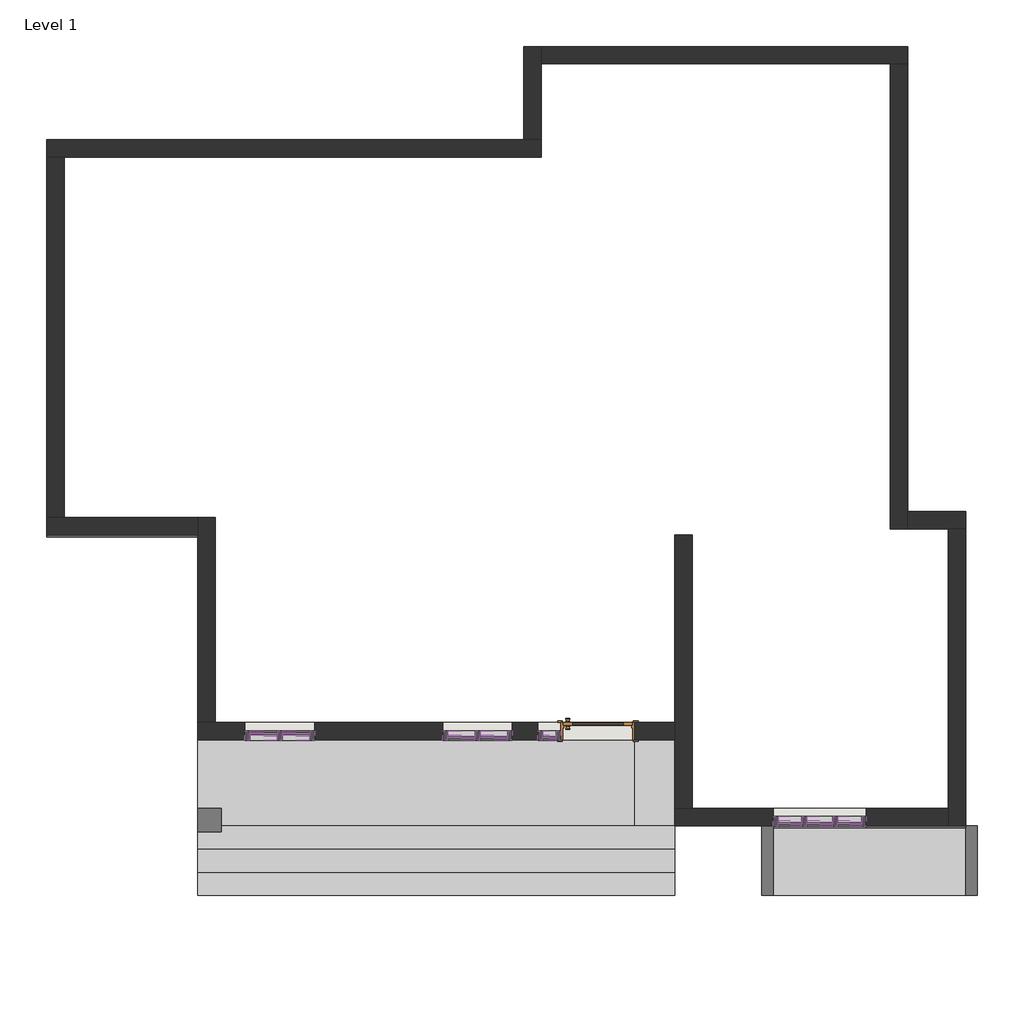
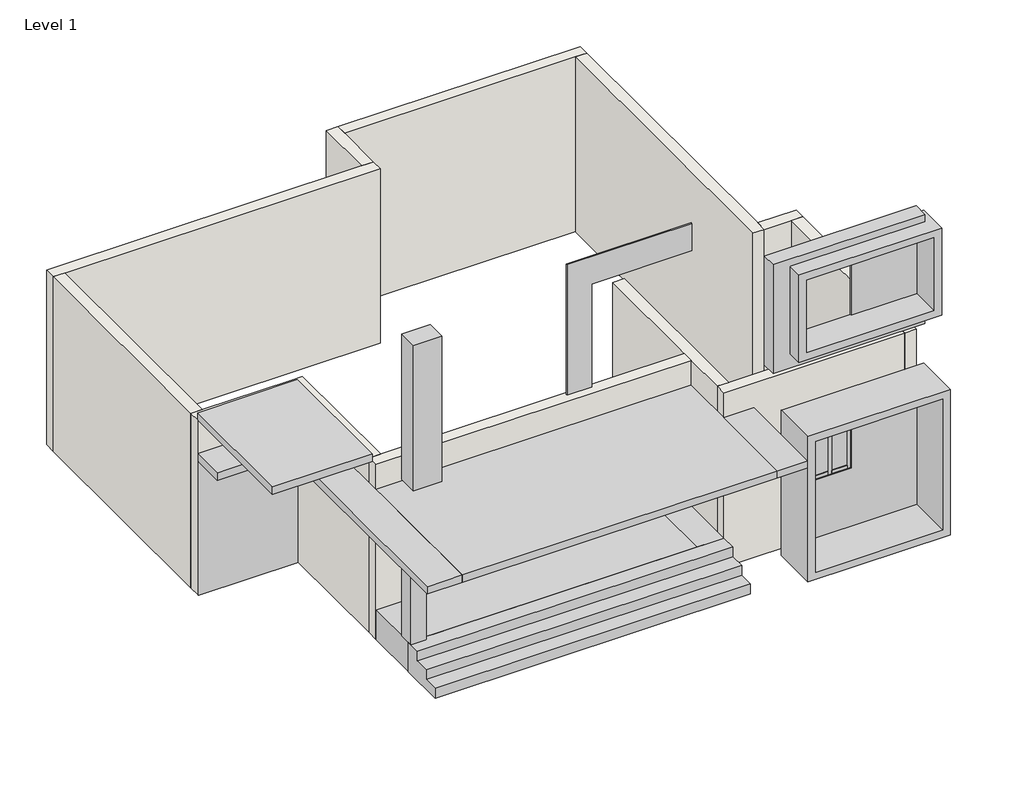
# One storey: 48 members, 16 plates, 12 walls, 1 door, 1 proxy.
"""IFC4 building model written with IfcOpenShell, lengths in millimetres."""

from ifc_helpers import new_model, si_unit, frame, origin, place, context, project, spatial, polyline, outline, extrude, faceted_brep, transform, mapped, element, save
from components import generic_models_1_generic_models_1_206d5355, door_3b97b8e7, member_2344d604, member_a0100b10, member_6c57b699, member_2c71ef08, member_843225dc, member_824a4a8d, member_ffd4c858, member_15823cb3, member_c6627131, member_d92184fb, member_69a911c1, member_f07b7441, member_5ad95953, member_f92b8aa2, member_ff1b7d8f, member_90750a43, member_7fd687a9, member_8e09d03a, system_panel_glazed_8f314941, system_panel_glazed_b220ba01, system_panel_glazed_f8f6f98b, system_panel_glazed_d1623790, system_panel_glazed_0360dae9, system_panel_glazed_809156e5, system_panel_glazed_ff0761ce, system_panel_glazed_bfcc9025

model = new_model("IFC4")

# Units and contexts
model_context = context("Model", 3, world=origin())
ifc_project = project(units=[si_unit("LENGTHUNIT", "METRE", prefix="MILLI")], contexts=[model_context])

# Site, building, storey
site = spatial("IfcSite", under=ifc_project)
building = spatial("IfcBuilding", under=site)
storey = spatial("IfcBuildingStorey", under=building, Name="Level 1", Elevation=0.0)

# Proxy
placement = place(None, origin())
generic_models_1_generic_models_1_shape = generic_models_1_generic_models_1_206d5355(model_context)
element("IfcBuildingElementProxy", 1, Name="Generic Models 1 : Generic Models 1", ObjectType="Generic Models 1 : Generic Models 1", at=placement, inside=storey, context=model_context, shape_type="MappedRepresentation", body=[
    mapped(generic_models_1_generic_models_1_shape, transform((0.0, 0.0, 0.0), x_axis=(1.0, 0.0, 0.0), y_axis=(0.0, 1.0, 0.0), z_axis=(0.0, 0.0, 1.0))),
])

# Door
door_shape = door_3b97b8e7(model_context)
element("IfcDoor", 2, ObjectType="Door-Interior-Single-1_Panel-Wood : 36\" x 84\"", at=placement, inside=storey, context=model_context, shape_type="MappedRepresentation", body=[
    mapped(door_shape, transform((-2625.1415113, 1605.7349631, 0.0), x_axis=(1.0, 0.0, 0.0), y_axis=(0.0, 1.0, 0.0), z_axis=(0.0, 0.0, 1.0))),
])

# Members
member_shape = member_2344d604(model_context)
element("IfcMember", 3, ObjectType="Rectangular Mullion : 1\" Square", at=placement, inside=storey, context=model_context, shape_type="MappedRepresentation", body=[
    mapped(member_shape, transform((-6397.0415113, 1545.4099631, 1676.4), x_axis=(0.0, 0.0, 1.0), y_axis=(0.0, -1.0, 0.0), z_axis=(1.0, 0.0, 0.0))),
])
element("IfcMember", 4, ObjectType="Rectangular Mullion : 1\" Square", at=placement, inside=storey, context=model_context, shape_type="MappedRepresentation", body=[
    mapped(member_shape, transform((-6822.4915113, 1545.4099631, 1676.4), x_axis=(0.0, 0.0, 1.0), y_axis=(0.0, -1.0, 0.0), z_axis=(1.0, 0.0, 0.0))),
])
element("IfcMember", 5, ObjectType="Rectangular Mullion : 1\" Square", at=placement, inside=storey, context=model_context, shape_type="MappedRepresentation", body=[
    mapped(member_shape, transform((-4593.6415113, 1545.4099631, 1676.4), x_axis=(0.0, 0.0, 1.0), y_axis=(0.0, 1.0, 0.0), z_axis=(-1.0, 0.0, 0.0))),
])
element("IfcMember", 6, ObjectType="Rectangular Mullion : 1\" Square", at=placement, inside=storey, context=model_context, shape_type="MappedRepresentation", body=[
    mapped(member_shape, transform((-4168.1915113, 1545.4099631, 1676.4), x_axis=(0.0, 0.0, 1.0), y_axis=(0.0, 1.0, 0.0), z_axis=(-1.0, 0.0, 0.0))),
])
member_2_shape = member_a0100b10(model_context)
element("IfcMember", 7, ObjectType="Rectangular Mullion : 1\" Square", at=placement, inside=storey, context=model_context, shape_type="MappedRepresentation", body=[
    mapped(member_2_shape, transform((-3349.0415113, 1545.4099631, 1701.8), x_axis=(0.0, 0.0, 1.0), y_axis=(0.0, 1.0, 0.0), z_axis=(-1.0, 0.0, 0.0))),
])
member_3_shape = member_6c57b699(model_context)
element("IfcMember", 8, ObjectType="Rectangular Mullion : 1\" Square", at=placement, inside=storey, context=model_context, shape_type="MappedRepresentation", body=[
    mapped(member_3_shape, transform((111.7084887, 421.4599631, 1625.6), x_axis=(0.0, 0.0, 1.0), y_axis=(0.0, 1.0, 0.0), z_axis=(-1.0, 0.0, 0.0))),
])
member_4_shape = member_2c71ef08(model_context)
element("IfcMember", 9, ObjectType="Rectangular Mullion : 1\" Square", at=placement, inside=storey, context=model_context, shape_type="MappedRepresentation", body=[
    mapped(member_4_shape, transform((-262.9415113, 421.4599631, 1625.6), x_axis=(0.0, 0.0, 1.0), y_axis=(0.0, 1.0, 0.0), z_axis=(-1.0, 0.0, 0.0))),
])
element("IfcMember", 10, ObjectType="Rectangular Mullion : 1\" Square", at=placement, inside=storey, context=model_context, shape_type="MappedRepresentation", body=[
    mapped(member_4_shape, transform((518.1084887, 421.4599631, 1625.6), x_axis=(0.0, 0.0, 1.0), y_axis=(0.0, 1.0, 0.0), z_axis=(-1.0, 0.0, 0.0))),
])
member_5_shape = member_843225dc(model_context)
element("IfcMember", 11, ObjectType="Rectangular Mullion : 2.5\" x 5\" rectangular", at=placement, inside=storey, context=model_context, shape_type="MappedRepresentation", body=[
    mapped(member_5_shape, transform((-6397.0415113, 1545.4099631, 2133.6), x_axis=(0.0, 0.0, 1.0), y_axis=(0.0, -1.0, 0.0), z_axis=(1.0, 0.0, 0.0))),
])
element("IfcMember", 12, ObjectType="Rectangular Mullion : 2.5\" x 5\" rectangular", at=placement, inside=storey, context=model_context, shape_type="MappedRepresentation", body=[
    mapped(member_5_shape, transform((-6822.4915113, 1545.4099631, 2133.6), x_axis=(0.0, 0.0, 1.0), y_axis=(0.0, -1.0, 0.0), z_axis=(1.0, 0.0, 0.0))),
])
element("IfcMember", 13, ObjectType="Rectangular Mullion : 2.5\" x 5\" rectangular", at=placement, inside=storey, context=model_context, shape_type="MappedRepresentation", body=[
    mapped(member_5_shape, transform((-4593.6415113, 1545.4099631, 2133.6), x_axis=(0.0, 0.0, 1.0), y_axis=(0.0, 1.0, 0.0), z_axis=(-1.0, 0.0, 0.0))),
])
element("IfcMember", 14, ObjectType="Rectangular Mullion : 2.5\" x 5\" rectangular", at=placement, inside=storey, context=model_context, shape_type="MappedRepresentation", body=[
    mapped(member_5_shape, transform((-4168.1915113, 1545.4099631, 2133.6), x_axis=(0.0, 0.0, 1.0), y_axis=(0.0, 1.0, 0.0), z_axis=(-1.0, 0.0, 0.0))),
])
element("IfcMember", 15, ObjectType="Rectangular Mullion : 2.5\" x 5\" rectangular", at=placement, inside=storey, context=model_context, shape_type="MappedRepresentation", body=[
    mapped(member_5_shape, transform((-7184.4415113, 1545.4099631, 304.8), x_axis=(0.0, 0.0, -1.0), y_axis=(0.0, -1.0, 0.0), z_axis=(-1.0, 0.0, 0.0))),
])
element("IfcMember", 16, ObjectType="Rectangular Mullion : 2.5\" x 5\" rectangular", at=placement, inside=storey, context=model_context, shape_type="MappedRepresentation", body=[
    mapped(member_5_shape, transform((-6758.9915113, 1545.4099631, 304.8), x_axis=(0.0, 0.0, -1.0), y_axis=(0.0, -1.0, 0.0), z_axis=(-1.0, 0.0, 0.0))),
])
element("IfcMember", 17, ObjectType="Rectangular Mullion : 2.5\" x 5\" rectangular", at=placement, inside=storey, context=model_context, shape_type="MappedRepresentation", body=[
    mapped(member_5_shape, transform((-3806.2415113, 1545.4099631, 304.8), x_axis=(0.0, 0.0, -1.0), y_axis=(0.0, 1.0, 0.0), z_axis=(1.0, 0.0, 0.0))),
])
element("IfcMember", 18, ObjectType="Rectangular Mullion : 2.5\" x 5\" rectangular", at=placement, inside=storey, context=model_context, shape_type="MappedRepresentation", body=[
    mapped(member_5_shape, transform((-4231.6915113, 1545.4099631, 304.8), x_axis=(0.0, 0.0, -1.0), y_axis=(0.0, 1.0, 0.0), z_axis=(1.0, 0.0, 0.0))),
])
member_6_shape = member_824a4a8d(model_context)
element("IfcMember", 19, ObjectType="Rectangular Mullion : 2.5\" x 5\" rectangular", at=placement, inside=storey, context=model_context, shape_type="MappedRepresentation", body=[
    mapped(member_6_shape, transform((-6790.7415113, 1545.4099631, 304.8), x_axis=(1.0, 0.0, 0.0), y_axis=(0.0, -1.0, 0.0), z_axis=(0.0, 0.0, -1.0))),
])
element("IfcMember", 20, ObjectType="Rectangular Mullion : 2.5\" x 5\" rectangular", at=placement, inside=storey, context=model_context, shape_type="MappedRepresentation", body=[
    mapped(member_6_shape, transform((-4199.9415113, 1545.4099631, 304.8), x_axis=(-1.0, 0.0, 0.0), y_axis=(0.0, 1.0, 0.0), z_axis=(0.0, 0.0, -1.0))),
])
member_7_shape = member_ffd4c858(model_context)
element("IfcMember", 21, ObjectType="Rectangular Mullion : 2.5\" x 5\" rectangular", at=placement, inside=storey, context=model_context, shape_type="MappedRepresentation", body=[
    mapped(member_7_shape, transform((-6790.7415113, 1545.4099631, 1676.4), x_axis=(1.0, 0.0, 0.0), y_axis=(0.0, -1.0, 0.0), z_axis=(0.0, 0.0, -1.0))),
])
element("IfcMember", 22, ObjectType="Rectangular Mullion : 2.5\" x 5\" rectangular", at=placement, inside=storey, context=model_context, shape_type="MappedRepresentation", body=[
    mapped(member_7_shape, transform((-4199.9415113, 1545.4099631, 1676.4), x_axis=(-1.0, 0.0, 0.0), y_axis=(0.0, 1.0, 0.0), z_axis=(0.0, 0.0, -1.0))),
])
member_8_shape = member_15823cb3(model_context)
element("IfcMember", 23, ObjectType="Rectangular Mullion : 2.5\" x 5\" rectangular", at=placement, inside=storey, context=model_context, shape_type="MappedRepresentation", body=[
    mapped(member_8_shape, transform((-7247.9415113, 1545.4099631, 2133.6), x_axis=(-1.0, 0.0, 0.0), y_axis=(0.0, -1.0, 0.0), z_axis=(0.0, 0.0, 1.0))),
])
element("IfcMember", 24, ObjectType="Rectangular Mullion : 2.5\" x 5\" rectangular", at=placement, inside=storey, context=model_context, shape_type="MappedRepresentation", body=[
    mapped(member_8_shape, transform((-3742.7415113, 1545.4099631, 2133.6), x_axis=(1.0, 0.0, 0.0), y_axis=(0.0, 1.0, 0.0), z_axis=(0.0, 0.0, 1.0))),
])
member_9_shape = member_c6627131(model_context)
element("IfcMember", 25, ObjectType="Rectangular Mullion : 2.5\" x 5\" rectangular", at=placement, inside=storey, context=model_context, shape_type="MappedRepresentation", body=[
    mapped(member_9_shape, transform((-6333.5415113, 1545.4099631, 304.8), x_axis=(1.0, 0.0, 0.0), y_axis=(0.0, -1.0, 0.0), z_axis=(0.0, 0.0, -1.0))),
])
element("IfcMember", 26, ObjectType="Rectangular Mullion : 2.5\" x 5\" rectangular", at=placement, inside=storey, context=model_context, shape_type="MappedRepresentation", body=[
    mapped(member_9_shape, transform((-4657.1415113, 1545.4099631, 304.8), x_axis=(-1.0, 0.0, 0.0), y_axis=(0.0, 1.0, 0.0), z_axis=(0.0, 0.0, -1.0))),
])
element("IfcMember", 27, ObjectType="Rectangular Mullion : 2.5\" x 5\" rectangular", at=placement, inside=storey, context=model_context, shape_type="MappedRepresentation", body=[
    mapped(member_8_shape, transform((-6333.5415113, 1545.4099631, 1676.4), x_axis=(1.0, 0.0, 0.0), y_axis=(0.0, -1.0, 0.0), z_axis=(0.0, 0.0, -1.0))),
])
element("IfcMember", 28, ObjectType="Rectangular Mullion : 2.5\" x 5\" rectangular", at=placement, inside=storey, context=model_context, shape_type="MappedRepresentation", body=[
    mapped(member_8_shape, transform((-4657.1415113, 1545.4099631, 1676.4), x_axis=(-1.0, 0.0, 0.0), y_axis=(0.0, 1.0, 0.0), z_axis=(0.0, 0.0, -1.0))),
])
element("IfcMember", 29, ObjectType="Rectangular Mullion : 2.5\" x 5\" rectangular", at=placement, inside=storey, context=model_context, shape_type="MappedRepresentation", body=[
    mapped(member_9_shape, transform((-7247.9415113, 1545.4099631, 1676.4), x_axis=(-1.0, 0.0, 0.0), y_axis=(0.0, -1.0, 0.0), z_axis=(0.0, 0.0, 1.0))),
])
element("IfcMember", 30, ObjectType="Rectangular Mullion : 2.5\" x 5\" rectangular", at=placement, inside=storey, context=model_context, shape_type="MappedRepresentation", body=[
    mapped(member_9_shape, transform((-3742.7415113, 1545.4099631, 1676.4), x_axis=(1.0, 0.0, 0.0), y_axis=(0.0, 1.0, 0.0), z_axis=(0.0, 0.0, 1.0))),
])
member_10_shape = member_d92184fb(model_context)
element("IfcMember", 31, ObjectType="Rectangular Mullion : 2.5\" x 5\" rectangular", at=placement, inside=storey, context=model_context, shape_type="MappedRepresentation", body=[
    mapped(member_10_shape, transform((-3349.0415113, 1545.4099631, 2133.6), x_axis=(0.0, 0.0, 1.0), y_axis=(0.0, 1.0, 0.0), z_axis=(-1.0, 0.0, 0.0))),
])
element("IfcMember", 32, ObjectType="Rectangular Mullion : 2.5\" x 5\" rectangular", at=placement, inside=storey, context=model_context, shape_type="MappedRepresentation", body=[
    mapped(member_10_shape, transform((-3171.2415113, 1545.4099631, 304.8), x_axis=(0.0, 0.0, -1.0), y_axis=(0.0, 1.0, 0.0), z_axis=(1.0, 0.0, 0.0))),
])
member_11_shape = member_69a911c1(model_context)
element("IfcMember", 33, ObjectType="Rectangular Mullion : 2.5\" x 5\" rectangular", at=placement, inside=storey, context=model_context, shape_type="MappedRepresentation", body=[
    mapped(member_11_shape, transform((-3107.7415113, 1545.4099631, 2133.6), x_axis=(1.0, 0.0, 0.0), y_axis=(0.0, 1.0, 0.0), z_axis=(0.0, 0.0, 1.0))),
])
member_12_shape = member_f07b7441(model_context)
element("IfcMember", 34, ObjectType="Rectangular Mullion : 2.5\" x 5\" rectangular", at=placement, inside=storey, context=model_context, shape_type="MappedRepresentation", body=[
    mapped(member_12_shape, transform((-3412.5415113, 1545.4099631, 304.8), x_axis=(-1.0, 0.0, 0.0), y_axis=(0.0, 1.0, 0.0), z_axis=(0.0, 0.0, -1.0))),
])
element("IfcMember", 35, ObjectType="Rectangular Mullion : 2.5\" x 5\" rectangular", at=placement, inside=storey, context=model_context, shape_type="MappedRepresentation", body=[
    mapped(member_11_shape, transform((-3412.5415113, 1545.4099631, 1701.8), x_axis=(-1.0, 0.0, 0.0), y_axis=(0.0, 1.0, 0.0), z_axis=(0.0, 0.0, -1.0))),
])
element("IfcMember", 36, ObjectType="Rectangular Mullion : 2.5\" x 5\" rectangular", at=placement, inside=storey, context=model_context, shape_type="MappedRepresentation", body=[
    mapped(member_12_shape, transform((-3107.7415113, 1545.4099631, 1701.8), x_axis=(1.0, 0.0, 0.0), y_axis=(0.0, 1.0, 0.0), z_axis=(0.0, 0.0, 1.0))),
])
member_13_shape = member_5ad95953(model_context)
element("IfcMember", 37, ObjectType="Rectangular Mullion : 2.5\" x 5\" rectangular", at=placement, inside=storey, context=model_context, shape_type="MappedRepresentation", body=[
    mapped(member_13_shape, transform((-262.9415113, 421.4599631, 2133.6), x_axis=(0.0, 0.0, 1.0), y_axis=(0.0, 1.0, 0.0), z_axis=(-1.0, 0.0, 0.0))),
])
element("IfcMember", 38, ObjectType="Rectangular Mullion : 2.5\" x 5\" rectangular", at=placement, inside=storey, context=model_context, shape_type="MappedRepresentation", body=[
    mapped(member_13_shape, transform((518.1084887, 421.4599631, 2133.6), x_axis=(0.0, 0.0, 1.0), y_axis=(0.0, 1.0, 0.0), z_axis=(-1.0, 0.0, 0.0))),
])
element("IfcMember", 39, ObjectType="Rectangular Mullion : 2.5\" x 5\" rectangular", at=placement, inside=storey, context=model_context, shape_type="MappedRepresentation", body=[
    mapped(member_13_shape, transform((829.2584887, 421.4599631, 609.6), x_axis=(0.0, 0.0, -1.0), y_axis=(0.0, 1.0, 0.0), z_axis=(1.0, 0.0, 0.0))),
])
element("IfcMember", 40, ObjectType="Rectangular Mullion : 2.5\" x 5\" rectangular", at=placement, inside=storey, context=model_context, shape_type="MappedRepresentation", body=[
    mapped(member_13_shape, transform((48.2084887, 421.4599631, 609.6), x_axis=(0.0, 0.0, -1.0), y_axis=(0.0, 1.0, 0.0), z_axis=(1.0, 0.0, 0.0))),
])
member_14_shape = member_f92b8aa2(model_context)
element("IfcMember", 41, ObjectType="Rectangular Mullion : 2.5\" x 5\" rectangular", at=placement, inside=storey, context=model_context, shape_type="MappedRepresentation", body=[
    mapped(member_14_shape, transform((79.9584887, 421.4599631, 609.6), x_axis=(-1.0, 0.0, 0.0), y_axis=(0.0, 1.0, 0.0), z_axis=(0.0, 0.0, -1.0))),
])
element("IfcMember", 42, ObjectType="Rectangular Mullion : 2.5\" x 5\" rectangular", at=placement, inside=storey, context=model_context, shape_type="MappedRepresentation", body=[
    mapped(member_14_shape, transform((486.3584887, 421.4599631, 609.6), x_axis=(-1.0, 0.0, 0.0), y_axis=(0.0, 1.0, 0.0), z_axis=(0.0, 0.0, -1.0))),
])
member_15_shape = member_ff1b7d8f(model_context)
element("IfcMember", 43, ObjectType="Rectangular Mullion : 2.5\" x 5\" rectangular", at=placement, inside=storey, context=model_context, shape_type="MappedRepresentation", body=[
    mapped(member_15_shape, transform((454.6084887, 421.4599631, 609.6), x_axis=(0.0, 0.0, -1.0), y_axis=(0.0, 1.0, 0.0), z_axis=(1.0, 0.0, 0.0))),
])
element("IfcMember", 44, ObjectType="Rectangular Mullion : 2.5\" x 5\" rectangular", at=placement, inside=storey, context=model_context, shape_type="MappedRepresentation", body=[
    mapped(member_15_shape, transform((111.7084887, 421.4599631, 2133.6), x_axis=(0.0, 0.0, 1.0), y_axis=(0.0, 1.0, 0.0), z_axis=(-1.0, 0.0, 0.0))),
])
member_16_shape = member_90750a43(model_context)
element("IfcMember", 45, ObjectType="Rectangular Mullion : 2.5\" x 5\" rectangular", at=placement, inside=storey, context=model_context, shape_type="MappedRepresentation", body=[
    mapped(member_16_shape, transform((79.9584887, 421.4599631, 1625.6), x_axis=(-1.0, 0.0, 0.0), y_axis=(0.0, 1.0, 0.0), z_axis=(0.0, 0.0, -1.0))),
])
element("IfcMember", 46, ObjectType="Rectangular Mullion : 2.5\" x 5\" rectangular", at=placement, inside=storey, context=model_context, shape_type="MappedRepresentation", body=[
    mapped(member_16_shape, transform((486.3584887, 421.4599631, 1625.6), x_axis=(-1.0, 0.0, 0.0), y_axis=(0.0, 1.0, 0.0), z_axis=(0.0, 0.0, -1.0))),
])
member_17_shape = member_7fd687a9(model_context)
element("IfcMember", 47, ObjectType="Rectangular Mullion : 2.5\" x 5\" rectangular", at=placement, inside=storey, context=model_context, shape_type="MappedRepresentation", body=[
    mapped(member_17_shape, transform((892.7584887, 421.4599631, 2133.6), x_axis=(1.0, 0.0, 0.0), y_axis=(0.0, 1.0, 0.0), z_axis=(0.0, 0.0, 1.0))),
])
member_18_shape = member_8e09d03a(model_context)
element("IfcMember", 48, ObjectType="Rectangular Mullion : 2.5\" x 5\" rectangular", at=placement, inside=storey, context=model_context, shape_type="MappedRepresentation", body=[
    mapped(member_18_shape, transform((-326.4415113, 421.4599631, 609.6), x_axis=(-1.0, 0.0, 0.0), y_axis=(0.0, 1.0, 0.0), z_axis=(0.0, 0.0, -1.0))),
])
element("IfcMember", 49, ObjectType="Rectangular Mullion : 2.5\" x 5\" rectangular", at=placement, inside=storey, context=model_context, shape_type="MappedRepresentation", body=[
    mapped(member_17_shape, transform((-326.4415113, 421.4599631, 1625.6), x_axis=(-1.0, 0.0, 0.0), y_axis=(0.0, 1.0, 0.0), z_axis=(0.0, 0.0, -1.0))),
])
element("IfcMember", 50, ObjectType="Rectangular Mullion : 2.5\" x 5\" rectangular", at=placement, inside=storey, context=model_context, shape_type="MappedRepresentation", body=[
    mapped(member_18_shape, transform((892.7584887, 421.4599631, 1625.6), x_axis=(1.0, 0.0, 0.0), y_axis=(0.0, 1.0, 0.0), z_axis=(0.0, 0.0, 1.0))),
])

# Plates
system_panel_glazed_shape = system_panel_glazed_8f314941(model_context)
element("IfcPlate", 51, ObjectType="System Panel : Glazed", at=placement, inside=storey, context=model_context, shape_type="MappedRepresentation", body=[
    mapped(system_panel_glazed_shape, transform((-3987.2165113, 1545.4099631, 368.3), x_axis=(-1.0, 0.0, 0.0), y_axis=(0.0, -1.0, 0.0), z_axis=(0.0, 0.0, 1.0))),
])
element("IfcPlate", 52, ObjectType="System Panel : Glazed", at=placement, inside=storey, context=model_context, shape_type="MappedRepresentation", body=[
    mapped(system_panel_glazed_shape, transform((-7003.4665113, 1545.4099631, 368.3), x_axis=(1.0, 0.0, 0.0), y_axis=(0.0, 1.0, 0.0), z_axis=(0.0, 0.0, 1.0))),
])
element("IfcPlate", 53, ObjectType="System Panel : Glazed", at=placement, inside=storey, context=model_context, shape_type="MappedRepresentation", body=[
    mapped(system_panel_glazed_shape, transform((-6578.0165113, 1545.4099631, 368.3), x_axis=(1.0, 0.0, 0.0), y_axis=(0.0, 1.0, 0.0), z_axis=(0.0, 0.0, 1.0))),
])
element("IfcPlate", 54, ObjectType="System Panel : Glazed", at=placement, inside=storey, context=model_context, shape_type="MappedRepresentation", body=[
    mapped(system_panel_glazed_shape, transform((-4412.6665113, 1545.4099631, 368.3), x_axis=(-1.0, 0.0, 0.0), y_axis=(0.0, -1.0, 0.0), z_axis=(0.0, 0.0, 1.0))),
])
system_panel_glazed_2_shape = system_panel_glazed_b220ba01(model_context)
element("IfcPlate", 55, ObjectType="System Panel : Glazed", at=placement, inside=storey, context=model_context, shape_type="MappedRepresentation", body=[
    mapped(system_panel_glazed_2_shape, transform((-7003.4665113, 1545.4099631, 1676.4), x_axis=(1.0, 0.0, 0.0), y_axis=(0.0, 1.0, 0.0), z_axis=(0.0, 0.0, 1.0))),
])
element("IfcPlate", 56, ObjectType="System Panel : Glazed", at=placement, inside=storey, context=model_context, shape_type="MappedRepresentation", body=[
    mapped(system_panel_glazed_2_shape, transform((-6578.0165113, 1545.4099631, 1676.4), x_axis=(1.0, 0.0, 0.0), y_axis=(0.0, 1.0, 0.0), z_axis=(0.0, 0.0, 1.0))),
])
element("IfcPlate", 57, ObjectType="System Panel : Glazed", at=placement, inside=storey, context=model_context, shape_type="MappedRepresentation", body=[
    mapped(system_panel_glazed_2_shape, transform((-3987.2165113, 1545.4099631, 1676.4), x_axis=(-1.0, 0.0, 0.0), y_axis=(0.0, -1.0, 0.0), z_axis=(0.0, 0.0, 1.0))),
])
element("IfcPlate", 58, ObjectType="System Panel : Glazed", at=placement, inside=storey, context=model_context, shape_type="MappedRepresentation", body=[
    mapped(system_panel_glazed_2_shape, transform((-4412.6665113, 1545.4099631, 1676.4), x_axis=(-1.0, 0.0, 0.0), y_axis=(0.0, -1.0, 0.0), z_axis=(0.0, 0.0, 1.0))),
])
system_panel_glazed_3_shape = system_panel_glazed_f8f6f98b(model_context)
element("IfcPlate", 59, ObjectType="System Panel : Glazed", at=placement, inside=storey, context=model_context, shape_type="MappedRepresentation", body=[
    mapped(system_panel_glazed_3_shape, transform((-3260.1415113, 1545.4099631, 368.3), x_axis=(-1.0, 0.0, 0.0), y_axis=(0.0, -1.0, 0.0), z_axis=(0.0, 0.0, 1.0))),
])
system_panel_glazed_4_shape = system_panel_glazed_d1623790(model_context)
element("IfcPlate", 60, ObjectType="System Panel : Glazed", at=placement, inside=storey, context=model_context, shape_type="MappedRepresentation", body=[
    mapped(system_panel_glazed_4_shape, transform((-3260.1415113, 1545.4099631, 1701.8), x_axis=(-1.0, 0.0, 0.0), y_axis=(0.0, -1.0, 0.0), z_axis=(0.0, 0.0, 1.0))),
])
system_panel_glazed_5_shape = system_panel_glazed_0360dae9(model_context)
element("IfcPlate", 61, ObjectType="System Panel : Glazed", at=placement, inside=storey, context=model_context, shape_type="MappedRepresentation", body=[
    mapped(system_panel_glazed_5_shape, transform((673.6834887, 421.4599631, 673.1), x_axis=(-1.0, 0.0, 0.0), y_axis=(0.0, -1.0, 0.0), z_axis=(0.0, 0.0, 1.0))),
])
element("IfcPlate", 62, ObjectType="System Panel : Glazed", at=placement, inside=storey, context=model_context, shape_type="MappedRepresentation", body=[
    mapped(system_panel_glazed_5_shape, transform((-107.3665113, 421.4599631, 673.1), x_axis=(-1.0, 0.0, 0.0), y_axis=(0.0, -1.0, 0.0), z_axis=(0.0, 0.0, 1.0))),
])
system_panel_glazed_6_shape = system_panel_glazed_809156e5(model_context)
element("IfcPlate", 63, ObjectType="System Panel : Glazed", at=placement, inside=storey, context=model_context, shape_type="MappedRepresentation", body=[
    mapped(system_panel_glazed_6_shape, transform((283.1584887, 421.4599631, 673.1), x_axis=(-1.0, 0.0, 0.0), y_axis=(0.0, -1.0, 0.0), z_axis=(0.0, 0.0, 1.0))),
])
system_panel_glazed_7_shape = system_panel_glazed_ff0761ce(model_context)
element("IfcPlate", 64, ObjectType="System Panel : Glazed", at=placement, inside=storey, context=model_context, shape_type="MappedRepresentation", body=[
    mapped(system_panel_glazed_7_shape, transform((673.6834887, 421.4599631, 1625.6), x_axis=(-1.0, 0.0, 0.0), y_axis=(0.0, -1.0, 0.0), z_axis=(0.0, 0.0, 1.0))),
])
element("IfcPlate", 65, ObjectType="System Panel : Glazed", at=placement, inside=storey, context=model_context, shape_type="MappedRepresentation", body=[
    mapped(system_panel_glazed_7_shape, transform((-107.3665113, 421.4599631, 1625.6), x_axis=(-1.0, 0.0, 0.0), y_axis=(0.0, -1.0, 0.0), z_axis=(0.0, 0.0, 1.0))),
])
system_panel_glazed_8_shape = system_panel_glazed_bfcc9025(model_context)
element("IfcPlate", 66, ObjectType="System Panel : Glazed", at=placement, inside=storey, context=model_context, shape_type="MappedRepresentation", body=[
    mapped(system_panel_glazed_8_shape, transform((283.1584887, 421.4599631, 1625.6), x_axis=(-1.0, 0.0, 0.0), y_axis=(0.0, -1.0, 0.0), z_axis=(0.0, 0.0, 1.0))),
])

# Walls
element("IfcWall", 67, ObjectType="9\" wall", at=placement, inside=storey, context=model_context, shape_type="Brep", body=[
    faceted_brep([(-9845.0915113, 9127.3099631, -609.6), (-9616.4915113, 9127.3099631, -609.6), (-3368.0915113, 9127.3099631, -609.6), (-3368.0915113, 9127.3099631, 3048.0), (-9616.4915113, 9127.3099631, 3048.0), (-9845.0915113, 9127.3099631, 3048.0), (-9845.0915113, 9355.9099631, -609.6), (-9845.0915113, 9355.9099631, 3048.0), (-3596.6915113, 9355.9099631, 3048.0), (-3368.0915113, 9355.9099631, 3048.0), (-3368.0915113, 9355.9099631, -609.6), (-3596.6915113, 9355.9099631, -609.6)], [[[0, 1, 2, 3, 4, 5]], [[6, 7, 8, 9, 10, 11]], [[2, 1, 0, 6, 11, 10]], [[5, 4, 3, 9, 8, 7]], [[3, 2, 10, 9]], [[0, 5, 7, 6]]]),
])
element("IfcWall", 68, ObjectType="9\" wall", at=placement, inside=storey, context=model_context, shape_type="Brep", body=[
    faceted_brep([(-3368.0915113, 9355.9099631, -609.6), (-3368.0915113, 10346.5099631, -609.6), (-3368.0915113, 10575.1099631, -609.6), (-3368.0915113, 10575.1099631, 3048.0), (-3368.0915113, 10346.5099631, 3048.0), (-3368.0915113, 9355.9099631, 3048.0), (-3596.6915113, 9355.9099631, -609.6), (-3596.6915113, 9355.9099631, 3048.0), (-3596.6915113, 10575.1099631, 3048.0), (-3596.6915113, 10575.1099631, -609.6)], [[[0, 1, 2, 3, 4, 5]], [[6, 7, 8, 9]], [[2, 1, 0, 6, 9]], [[5, 4, 3, 8, 7]], [[0, 5, 7, 6]], [[3, 2, 9, 8]]]),
])
element("IfcWall", 69, ObjectType="9\" wall", at=placement, inside=storey, context=model_context, shape_type="Brep", body=[
    faceted_brep([(-3368.0915113, 10346.5099631, -609.6), (1203.9084887, 10346.5099631, -609.6), (1432.5084887, 10346.5099631, -609.6), (1432.5084887, 10346.5099631, 3048.0), (1203.9084887, 10346.5099631, 3048.0), (-3368.0915113, 10346.5099631, 3048.0), (-3368.0915113, 10575.1099631, -609.6), (-3368.0915113, 10575.1099631, 3048.0), (1432.5084887, 10575.1099631, 3048.0), (1432.5084887, 10575.1099631, -609.6)], [[[0, 1, 2, 3, 4, 5]], [[6, 7, 8, 9]], [[2, 1, 0, 6, 9]], [[5, 4, 3, 8, 7]], [[0, 5, 7, 6]], [[3, 2, 9, 8]]]),
])
element("IfcWall", 70, ObjectType="9\" wall", at=placement, inside=storey, context=model_context, shape_type="Brep", body=[
    faceted_brep([(1203.9084887, 10346.5099631, -609.6), (1203.9084887, 4250.5099631, -609.6), (1203.9084887, 4250.5099631, 3048.0), (1203.9084887, 10346.5099631, 3048.0), (1432.5084887, 10346.5099631, -609.6), (1432.5084887, 10346.5099631, 3048.0), (1432.5084887, 4479.1099631, 3048.0), (1432.5084887, 4250.5099631, 3048.0), (1432.5084887, 4250.5099631, -609.6), (1432.5084887, 4479.1099631, -609.6)], [[[0, 1, 2, 3]], [[4, 5, 6, 7, 8, 9]], [[1, 0, 4, 9, 8]], [[3, 2, 7, 6, 5]], [[0, 3, 5, 4]], [[2, 1, 8, 7]]]),
])
element("IfcWall", 71, ObjectType="9\" wall", at=placement, inside=storey, context=model_context, shape_type="Brep", body=[
    faceted_brep([(1432.5084887, 4250.5099631, -609.6), (1965.9084887, 4250.5099631, -609.6), (2194.5084887, 4250.5099631, -609.6), (2194.5084887, 4250.5099631, 3048.0), (1965.9084887, 4250.5099631, 3048.0), (1432.5084887, 4250.5099631, 3048.0), (1432.5084887, 4479.1099631, -609.6), (1432.5084887, 4479.1099631, 3048.0), (2194.5084887, 4479.1099631, 3048.0), (2194.5084887, 4479.1099631, -609.6)], [[[0, 1, 2, 3, 4, 5]], [[6, 7, 8, 9]], [[2, 1, 0, 6, 9]], [[5, 4, 3, 8, 7]], [[0, 5, 7, 6]], [[3, 2, 9, 8]]]),
])
element("IfcWall", 72, ObjectType="9\" wall", at=placement, inside=storey, context=model_context, shape_type="Brep", body=[
    faceted_brep([(1965.9084887, 4250.5099631, -609.6), (1965.9084887, 592.9099631, -609.6), (1965.9084887, 364.3099631, -609.6), (1965.9084887, 364.3099631, 3048.0), (1965.9084887, 592.9099631, 3048.0), (1965.9084887, 4250.5099631, 3048.0), (2194.5084887, 4250.5099631, -609.6), (2194.5084887, 4250.5099631, 3048.0), (2194.5084887, 364.3099631, 3048.0), (2194.5084887, 364.3099631, -609.6)], [[[0, 1, 2, 3, 4, 5]], [[6, 7, 8, 9]], [[2, 1, 0, 6, 9]], [[5, 4, 3, 8, 7]], [[0, 5, 7, 6]], [[3, 2, 9, 8]]]),
])
element("IfcWall", 73, ObjectType="9\" wall", at=placement, inside=storey, context=model_context, shape_type="Brep", body=[
    faceted_brep([(1965.9084887, 592.9099631, -609.6), (-1386.8915113, 592.9099631, -609.6), (-1615.4915113, 592.9099631, -609.6), (-1615.4915113, 592.9099631, 3048.0), (-1386.8915113, 592.9099631, 3048.0), (1965.9084887, 592.9099631, 3048.0), (892.7584887, 592.9099631, 609.6), (892.7584887, 592.9099631, 2133.6), (-326.4415113, 592.9099631, 2133.6), (-326.4415113, 592.9099631, 609.6), (-1615.4915113, 364.3099631, -609.6), (1965.9084887, 364.3099631, -609.6), (1965.9084887, 364.3099631, 3048.0), (-1615.4915113, 364.3099631, 3048.0), (-1615.4915113, 364.3099631, 2530.5713747), (892.7584887, 364.3099631, 2133.6), (892.7584887, 364.3099631, 609.6), (-326.4415113, 364.3099631, 609.6), (-326.4415113, 364.3099631, 2133.6)], [[[0, 1, 2, 3, 4, 5], [6, 7, 8, 9]], [[10, 11, 12, 13, 14], [15, 16, 17, 18]], [[2, 1, 0, 11, 10]], [[5, 4, 3, 13, 12]], [[0, 5, 12, 11]], [[6, 16, 15, 7]], [[7, 15, 18, 8]], [[8, 18, 17, 9]], [[16, 6, 9, 17]], [[2, 10, 14, 13, 3]]]),
])
element("IfcWall", 74, ObjectType="9\" wall", at=placement, inside=storey, context=model_context, shape_type="Brep", body=[
    faceted_brep([(-1386.8915113, 592.9099631, 3048.0), (-1386.8915113, 592.9099631, -609.6), (-1386.8915113, 4174.3099631, -609.6), (-1386.8915113, 4174.3099631, 3048.0), (-1615.4915113, 592.9099631, -609.6), (-1615.4915113, 592.9099631, 3048.0), (-1615.4915113, 1488.2599631, 3048.0), (-1615.4915113, 1716.8599631, 3048.0), (-1615.4915113, 4174.3099631, 3048.0), (-1615.4915113, 4174.3099631, -609.6), (-1615.4915113, 1716.8599631, -609.6), (-1615.4915113, 1488.2599631, -609.6)], [[[0, 1, 2, 3]], [[4, 5, 6, 7, 8, 9, 10, 11]], [[2, 1, 4, 11, 10, 9]], [[3, 2, 9, 8]], [[0, 3, 8, 7, 6, 5]], [[0, 5, 4, 1]]]),
])
element("IfcWall", 75, ObjectType="9\" wall", at=placement, inside=storey, context=model_context, shape_type="Brep", body=[
    faceted_brep([(-1615.4915113, 1716.8599631, -609.6), (-7635.2915113, 1716.8599631, -609.6), (-7863.8915113, 1716.8599631, -609.6), (-7863.8915113, 1716.8599631, 3048.0), (-7635.2915113, 1716.8599631, 3048.0), (-1615.4915113, 1716.8599631, 3048.0), (-2142.5415113, 1716.8599631, 0.0), (-2142.5415113, 1716.8599631, 2159.0), (-3107.7415113, 1716.8599631, 2159.0), (-3107.7415113, 1716.8599631, 2133.6), (-3412.5415113, 1716.8599631, 2133.6), (-3412.5415113, 1716.8599631, 304.8), (-3107.7415113, 1716.8599631, 304.8), (-3107.7415113, 1716.8599631, 0.0), (-7247.9415113, 1716.8599631, 2133.6), (-7247.9415113, 1716.8599631, 304.8), (-6333.5415113, 1716.8599631, 304.8), (-6333.5415113, 1716.8599631, 2133.6), (-3742.7415113, 1716.8599631, 304.8), (-3742.7415113, 1716.8599631, 2133.6), (-4657.1415113, 1716.8599631, 2133.6), (-4657.1415113, 1716.8599631, 304.8), (-7863.8915113, 1488.2599631, -609.6), (-1615.4915113, 1488.2599631, -609.6), (-1615.4915113, 1488.2599631, 3048.0), (-7863.8915113, 1488.2599631, 3048.0), (-7863.8915113, 1488.2599631, 2530.5713747), (-2142.5415113, 1488.2599631, 2159.0), (-2142.5415113, 1488.2599631, 0.0), (-3107.7415113, 1488.2599631, 0.0), (-3107.7415113, 1488.2599631, 304.8), (-3412.5415113, 1488.2599631, 304.8), (-3412.5415113, 1488.2599631, 2133.6), (-3107.7415113, 1488.2599631, 2133.6), (-3107.7415113, 1488.2599631, 2159.0), (-7247.9415113, 1488.2599631, 304.8), (-7247.9415113, 1488.2599631, 2133.6), (-6333.5415113, 1488.2599631, 2133.6), (-6333.5415113, 1488.2599631, 304.8), (-3742.7415113, 1488.2599631, 2133.6), (-3742.7415113, 1488.2599631, 304.8), (-4657.1415113, 1488.2599631, 304.8), (-4657.1415113, 1488.2599631, 2133.6)], [[[0, 1, 2, 3, 4, 5], [6, 7, 8, 9, 10, 11, 12, 13], [14, 15, 16, 17], [18, 19, 20, 21]], [[22, 23, 24, 25, 26], [27, 28, 29, 30, 31, 32, 33, 34], [35, 36, 37, 38], [39, 40, 41, 42]], [[2, 1, 0, 23, 22]], [[5, 4, 3, 25, 24]], [[0, 5, 24, 23]], [[6, 28, 27, 7]], [[7, 27, 34, 8]], [[29, 13, 12, 30]], [[8, 34, 33, 9]], [[28, 6, 13, 29]], [[35, 15, 14, 36]], [[36, 14, 17, 37]], [[37, 17, 16, 38]], [[15, 35, 38, 16]], [[39, 19, 18, 40]], [[19, 39, 42, 20]], [[20, 42, 41, 21]], [[40, 18, 21, 41]], [[32, 10, 9, 33]], [[10, 32, 31, 11]], [[11, 31, 30, 12]], [[2, 22, 26, 25, 3]]]),
])
element("IfcWall", 76, ObjectType="9\" wall", at=placement, inside=storey, context=model_context, shape_type="Brep", body=[
    faceted_brep([(-7635.2915113, 1716.8599631, 3048.0), (-7635.2915113, 1716.8599631, -609.6), (-7635.2915113, 4402.9099631, -609.6), (-7635.2915113, 4402.9099631, 3048.0), (-7863.8915113, 1716.8599631, -609.6), (-7863.8915113, 1716.8599631, 3048.0), (-7863.8915113, 4174.3099631, 3048.0), (-7863.8915113, 4402.9099631, 3048.0), (-7863.8915113, 4402.9099631, -609.6), (-7863.8915113, 4174.3099631, -609.6)], [[[0, 1, 2, 3]], [[4, 5, 6, 7, 8, 9]], [[2, 1, 4, 9, 8]], [[0, 3, 7, 6, 5]], [[3, 2, 8, 7]], [[0, 5, 4, 1]]]),
])
element("IfcWall", 77, ObjectType="9\" wall", at=placement, inside=storey, context=model_context, shape_type="Brep", body=[
    faceted_brep([(-7863.8915113, 4402.9099631, -609.6), (-9616.4915113, 4402.9099631, -609.6), (-9845.0915113, 4402.9099631, -609.6), (-9845.0915113, 4402.9099631, 3048.0), (-9616.4915113, 4402.9099631, 3048.0), (-7863.8915113, 4402.9099631, 3048.0), (-7863.8915113, 4174.3099631, -609.6), (-7863.8915113, 4174.3099631, 3048.0), (-9845.0915113, 4174.3099631, 3048.0), (-9845.0915113, 4174.3099631, -609.6)], [[[0, 1, 2, 3, 4, 5]], [[6, 7, 8, 9]], [[2, 1, 0, 6, 9]], [[5, 4, 3, 8, 7]], [[0, 5, 7, 6]], [[3, 2, 9, 8]]]),
])
element("IfcWall", 78, ObjectType="9\" wall", at=placement, inside=storey, context=model_context, shape_type="SweptSolid", body=[
    extrude(outline(polyline([(-9616.4915113, 9127.3099631), (-9616.4915113, 4402.9099631), (-9845.0915113, 4402.9099631), (-9845.0915113, 9127.3099631), (-9616.4915113, 9127.3099631)])), frame((0.0, 0.0, -609.6), z_axis=(0.0, 0.0, 1.0), x_axis=(1.0, 0.0, 0.0)), (0.0, 0.0, 1.0), 3657.6),
])

save(model, "model.ifc")

# Revit data of these elements
# Type "Door-Interior-Single-1_Panel-Wood : 36\" x 84\""
#   Type Mark = "8"
#   Assembly Code = "C1020300"
#   Analytic Construction = "Wooden"
#   Top Rail = 0' - 4 11/16"
#   Thickness = 0' - 1 3/8"
#   Thermal Resistance (R) = 2.5876 (h·ft²·°F)/BTU
#   Swing Angle [instance default] = 90.00°
#   Stiles = 0' - 4 3/4"
#   Rough Width = 3' - 2"
#   Rough Height = 7' - 1"
#   Height = 7' - 0"
#   Width = 3' - 0"
#   Heat Transfer Coefficient (U) = 0.3865 BTU/(h·ft²·°F)
#   Bottom Rail = 0' - 9 1/8"
#   Trim Material = Cherry
#   Panel Material = Cherry
#   Frame Material = Cherry
#   Door Handle Material = Aluminum
#   Visual Light Transmittance = 0
#   Solar Heat Gain Coefficient = 0
#   Wall Closure = (empty or 0)
#   Function = (empty or 0)
# Type "Rectangular Mullion : 1\" Square"
#   built-in parameter 1007304 = 0.0833333 (stored number, unit not read)
#   built-in parameter 1007301 = 0.0416667 (stored number, unit not read)
#   built-in parameter 1007300 = 0.0416667 (stored number, unit not read)
# Type "Rectangular Mullion : 2.5\" x 5\" rectangular"
#   built-in parameter 1007304 = 0.416667 (stored number, unit not read)
#   built-in parameter 1007301 = 0.104167 (stored number, unit not read)
#   built-in parameter 1007300 = 0.104167 (stored number, unit not read)
# Type "System Panel : Glazed"
#   Construction Type Id = "GSP4R"
#   Analytic Construction = "1/8 in Pilkington single glazing"
#   Visual Light Transmittance = 0.9
#   Solar Heat Gain Coefficient = 0.86
#   Heat Transfer Coefficient (U) = 1.18115 BTU/(h·ft²·°F)
#   Define Thermal Properties by = 1
# Type "9\" wall"
#   Assembly Code = "B2010"
#   Layers, outside or top first: 0' - 9" "Laminate, Ivory, Matte" (function 1)
# Element 1 (IfcBuildingElementProxy, "Generic Models 1 : Generic Models 1")
#   Phase Created = New Construction
#   Materials on its faces: "Laminate, Ivory, Matte", "Wood Planks"
# Element 2 (IfcDoor, "Door-Interior-Single-1_Panel-Wood : 36\" x 84\"")
#   Swing Angle = 90.00°
#   Phase Created = New Construction
#   Materials on its faces: "Cherry", "Aluminum"
# Elements 3, 4, 5, 6, 7, 8, 9, 10 (IfcMember, "Rectangular Mullion : 1\" Square")
#   Phase Created = New Construction
# Elements 11, 12, 13, 14, 15, 16, 17, 18, 19, 20, 21, 22, 23, 24, 25, 26, 27, 28, 29, 30, 31, 32, 33, 34, 35, 36, 37, 38, 39, 40, 41, 42, 43, 44, 45, 46, 47, 48, 49, 50 (IfcMember, "Rectangular Mullion : 2.5\" x 5\" rectangular")
#   Phase Created = New Construction
# Elements 51, 52, 53, 54, 55, 56, 57, 58, 59, 60, 61, 62, 63, 64, 65, 66 (IfcPlate, "System Panel : Glazed")
#   Phase Created = New Construction
#   Materials on its faces: "Glass"
# Elements 67, 68, 69, 70, 71, 72, 73, 74, 75, 76, 77, 78 (IfcWall, "9\" wall")
#   built-in parameter 1001111 = -2' - 0"
#   Top Offset = 0' - 0"
#   Base Offset = -2' - 0"
#   wall height = 12' - 0"
#   Phase Created = New Construction
#   Base Constraint = Level 1
#   Top Constraint = Level 2
#   Materials on its faces: "Laminate, Ivory, Matte"
# Materials
#   "Cherry": class "Wood", colour RGB 226 177 128, transparency 0, Description = "Prunus Serotina", Cost = 0
#   "Aluminum": class "Metal", colour RGB 247 247 247, transparency 0, Description = "Aluminum 6061", Cost = 0
#   "Laminate, Ivory, Matte": class "Plastic", colour RGB 247 247 239, transparency 0, Description = "Plastic Laminate - Ivory, Matte", Cost = 0
#   "Wood Planks": class "Wood", colour RGB 193 160 115, transparency 0, Description = "Physical material.", Cost = 0
#   "Glass": class "Glass", colour RGB 0 128 192, transparency 0.75, Description = "Soda Lime Glass", Cost = 0
